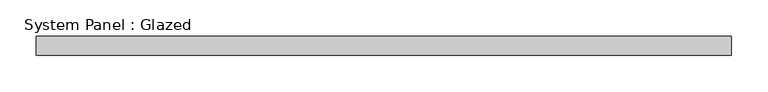
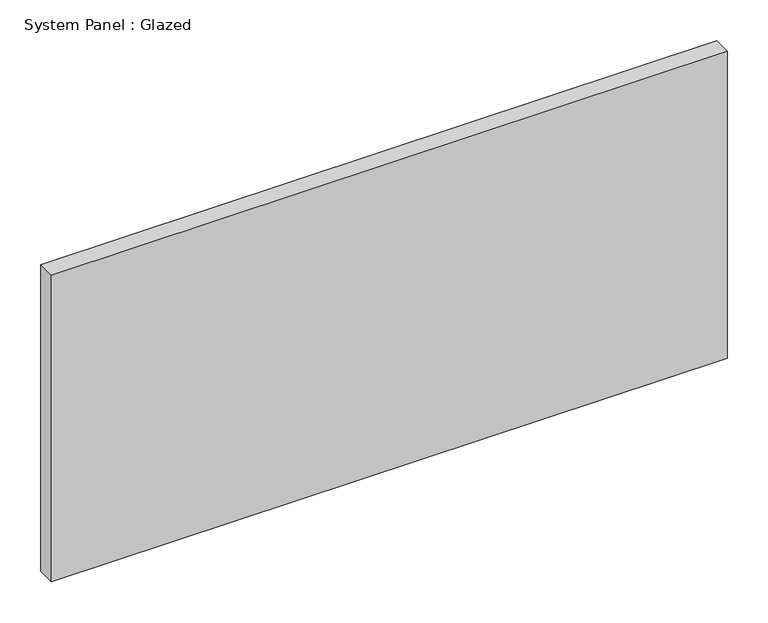
"""IFC4 building model written with IfcOpenShell, lengths in millimetres: plate geometry, System Panel : Glazed."""

from ifc_helpers import new_model, si_unit, origin, origin_with_axes, place, context, project, spatial, polyline, outline, extrude, source, transform, mapped, element, save


def system_panel_glazed_67d0ec78(model_context):
    return source(origin(), model_context, "Body", "SweptSolid", [
        extrude(outline(polyline([(476.25, 19.05), (-476.25, 19.05), (-476.25, 44.45), (476.25, 44.45), (476.25, 19.05)])), origin_with_axes(), (0.0, 0.0, 1.0), 457.2),
    ])


if __name__ == "__main__":
    model = new_model("IFC4")
    model_context = context("Model", 3, world=origin())
    ifc_project = project(units=[si_unit("LENGTHUNIT", "METRE", prefix="MILLI")], contexts=[model_context])
    site = spatial("IfcSite", under=ifc_project)
    building = spatial("IfcBuilding", under=site)
    placement = place(None, origin())
    system_panel_glazed_shape = system_panel_glazed_67d0ec78(model_context)
    element("IfcPlate", 1, ObjectType="System Panel : Glazed", at=placement, inside=building, context=model_context, shape_type="MappedRepresentation", body=[
        mapped(system_panel_glazed_shape, transform((0.0, 0.0, 0.0), x_axis=(1.0, 0.0, 0.0), y_axis=(0.0, 1.0, 0.0), z_axis=(0.0, 0.0, 1.0))),
    ])
    save(model, "model.ifc")

# Revit data of these elements
# Type "System Panel : Glazed"
#   Construction Type Id = "GSP4R"
#   Analytic Construction = "1/8 in Pilkington single glazing"
#   Visual Light Transmittance = 0.9
#   Solar Heat Gain Coefficient = 0.86
#   Heat Transfer Coefficient (U) = 1.18115 BTU/(h·ft²·°F)
#   Define Thermal Properties by = 1
# Element 1 (IfcPlate, "System Panel : Glazed")
#   Materials on its faces: "Glass"
# Materials
#   "Glass": class "Glass", colour RGB 0 128 192, transparency 0.75, Description = "Soda Lime Glass", Cost = 0
